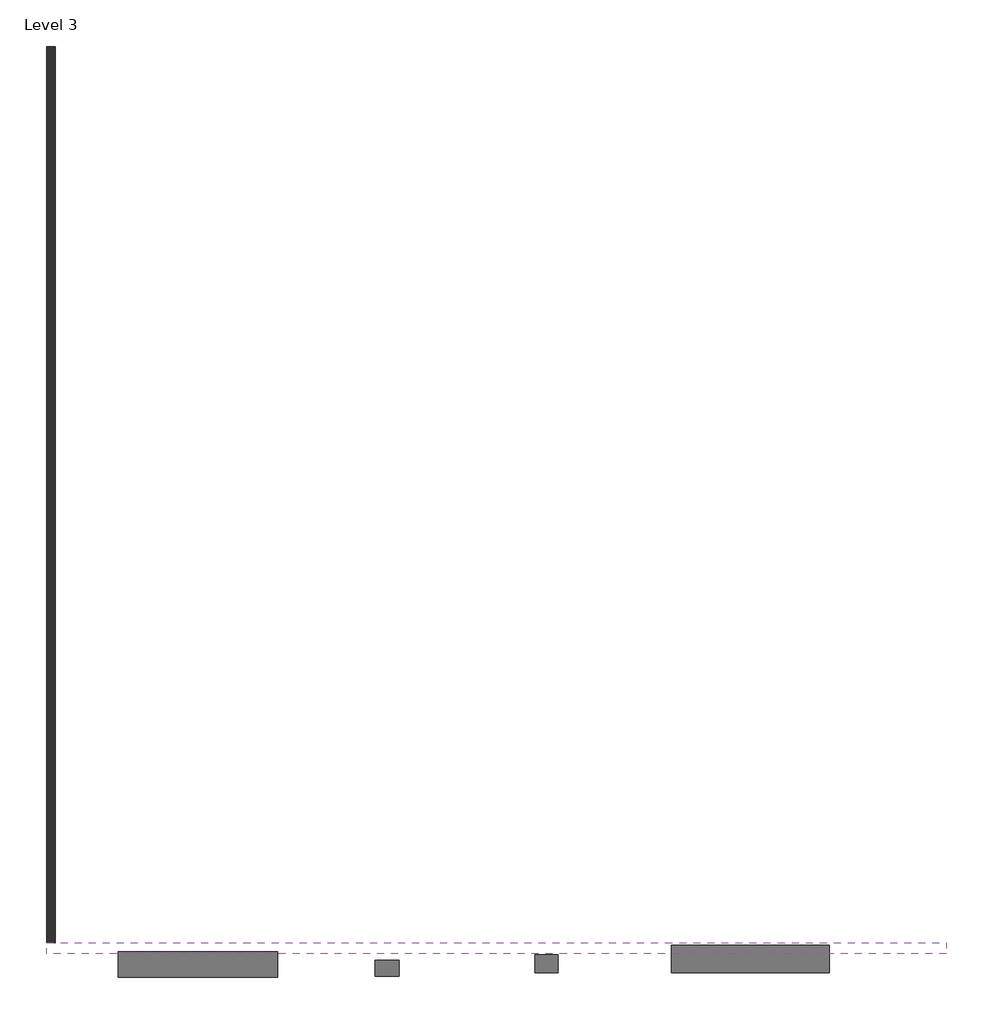
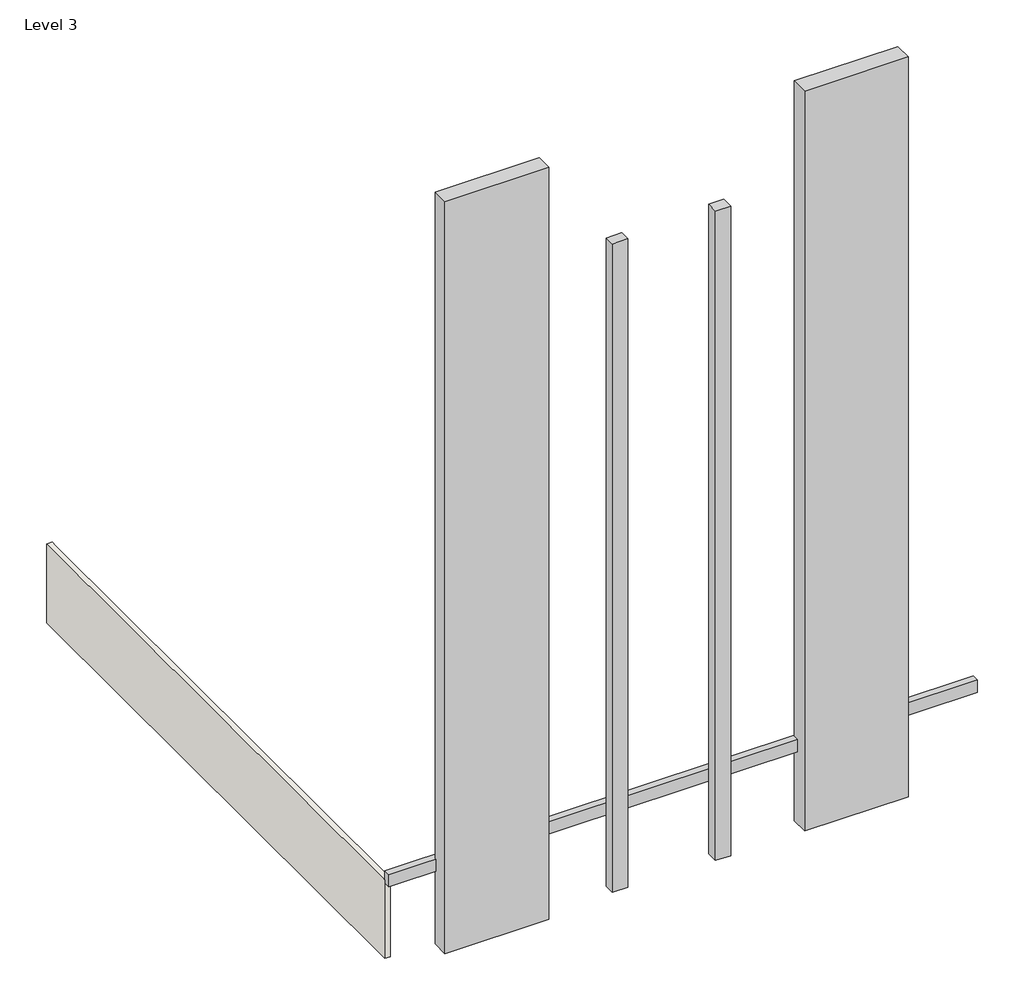
# One storey: 5 proxies, 1 wall.
"""IFC4 building model written with IfcOpenShell, lengths in millimetres."""

from ifc_helpers import new_model, si_unit, origin, place, context, project, spatial, faceted_brep, transform, mapped, element, save
from components import generic_models_11_generic_models_11_1ba3c33d, generic_models_12_generic_models_12_a991e301, generic_models_14_generic_models_14_86cac6df, generic_models_15_generic_models_15_a9d5df0f, generic_models_4_generic_models_4_7fc0937d

model = new_model("IFC4")

# Units and contexts
model_context = context("Model", 3, world=origin())
ifc_project = project(units=[si_unit("LENGTHUNIT", "METRE", prefix="MILLI")], contexts=[model_context])

# Site, building, storey
site = spatial("IfcSite", under=ifc_project)
building = spatial("IfcBuilding", under=site)
storey = spatial("IfcBuildingStorey", under=building, Name="Level 3", Elevation=3276.6)

# Proxies
placement = place(None, origin())
generic_models_11_generic_models_11_shape = generic_models_11_generic_models_11_1ba3c33d(model_context)
element("IfcBuildingElementProxy", 1, Name="Generic Models 11 : Generic Models 11", ObjectType="Generic Models 11 : Generic Models 11", at=placement, inside=storey, context=model_context, shape_type="MappedRepresentation", body=[
    mapped(generic_models_11_generic_models_11_shape, transform((0.0, 0.0, 0.0), x_axis=(1.0, 0.0, 0.0), y_axis=(0.0, 1.0, 0.0), z_axis=(0.0, 0.0, 1.0))),
])
generic_models_12_generic_models_12_shape = generic_models_12_generic_models_12_a991e301(model_context)
element("IfcBuildingElementProxy", 2, Name="Generic Models 12 : Generic Models 12", ObjectType="Generic Models 12 : Generic Models 12", at=placement, inside=storey, context=model_context, shape_type="MappedRepresentation", body=[
    mapped(generic_models_12_generic_models_12_shape, transform((0.0, 0.0, 0.0), x_axis=(1.0, 0.0, 0.0), y_axis=(0.0, 1.0, 0.0), z_axis=(0.0, 0.0, 1.0))),
])
generic_models_14_generic_models_14_shape = generic_models_14_generic_models_14_86cac6df(model_context)
element("IfcBuildingElementProxy", 3, Name="Generic Models 14 : Generic Models 14", ObjectType="Generic Models 14 : Generic Models 14", at=placement, inside=storey, context=model_context, shape_type="MappedRepresentation", body=[
    mapped(generic_models_14_generic_models_14_shape, transform((0.0, 0.0, 0.0), x_axis=(1.0, 0.0, 0.0), y_axis=(0.0, 1.0, 0.0), z_axis=(0.0, 0.0, 1.0))),
])
generic_models_15_generic_models_15_shape = generic_models_15_generic_models_15_a9d5df0f(model_context)
element("IfcBuildingElementProxy", 4, Name="Generic Models 15 : Generic Models 15", ObjectType="Generic Models 15 : Generic Models 15", at=placement, inside=storey, context=model_context, shape_type="MappedRepresentation", body=[
    mapped(generic_models_15_generic_models_15_shape, transform((0.0, 0.0, 0.0), x_axis=(1.0, 0.0, 0.0), y_axis=(0.0, 1.0, 0.0), z_axis=(0.0, 0.0, 1.0))),
])
generic_models_4_generic_models_4_shape = generic_models_4_generic_models_4_7fc0937d(model_context)
element("IfcBuildingElementProxy", 5, Name="Generic Models 4 : Generic Models 4", ObjectType="Generic Models 4 : Generic Models 4", at=placement, inside=storey, context=model_context, shape_type="MappedRepresentation", body=[
    mapped(generic_models_4_generic_models_4_shape, transform((0.0, 0.0, 0.0), x_axis=(1.0, 0.0, 0.0), y_axis=(0.0, 1.0, 0.0), z_axis=(0.0, 0.0, 1.0))),
])

# Wall
element("IfcWall", 6, ObjectType="outer wall", at=placement, inside=storey, context=model_context, shape_type="Brep", body=[
    faceted_brep([(-8731.5629849, -3682.5004242, 3276.6), (-8731.5629849, 17551.8995758, 3276.6), (-8731.5629849, 17755.0995758, 3276.6), (-8731.5629849, 17755.0995758, 6324.6), (-8731.5629849, 17551.8995758, 6324.6), (-8731.5629849, -3682.5004242, 6324.6), (-8934.7629849, -3682.5004242, 3276.6), (-8934.7629849, -3682.5004242, 6324.6), (-8934.7629849, 17755.0995758, 6324.6), (-8934.7629849, 17755.0995758, 3276.6), (-8934.7629849, 17551.8995758, 3276.6)], [[[0, 1, 2, 3, 4, 5]], [[6, 7, 8, 9, 10]], [[2, 1, 0, 6, 10, 9]], [[5, 4, 3, 8, 7]], [[0, 5, 7, 6]], [[3, 2, 9, 8]]]),
])

save(model, "model.ifc")

# Revit data of these elements
# Type "outer wall"
#   Assembly Code = "B2010"
#   Layers, outside or top first: 0' - 8" "Copper" (function 1)
# Element 1 (IfcBuildingElementProxy, "Generic Models 11 : Generic Models 11")
#   Phase Created = New Construction
# Element 2 (IfcBuildingElementProxy, "Generic Models 12 : Generic Models 12")
#   Phase Created = New Construction
# Element 3 (IfcBuildingElementProxy, "Generic Models 14 : Generic Models 14")
#   Phase Created = New Construction
# Element 4 (IfcBuildingElementProxy, "Generic Models 15 : Generic Models 15")
#   Phase Created = New Construction
# Element 5 (IfcBuildingElementProxy, "Generic Models 4 : Generic Models 4")
#   Phase Created = New Construction
# Element 6 (IfcWall, "outer wall")
#   Top Offset = 0' - 0"
#   Base Offset = 0' - 0"
#   Unconnected Height = 10' - 0"
#   wall height = 10' - 0"
#   Phase Created = New Construction
#   Base Constraint = Level 3
#   Materials on its faces: "Copper"
# Materials
#   "Copper": class "Metal", colour RGB 0 0 0, transparency 0, Description = "Copper, matte finish", Cost = 0
